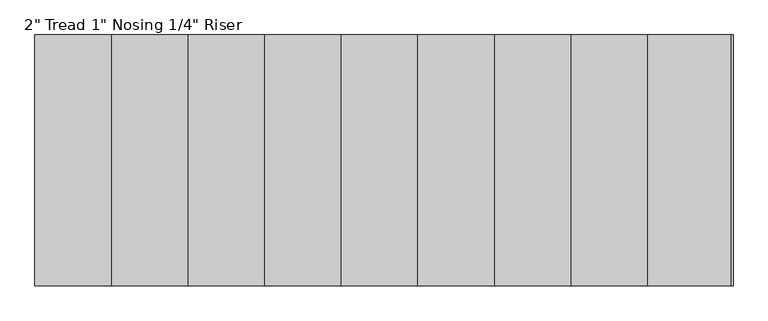
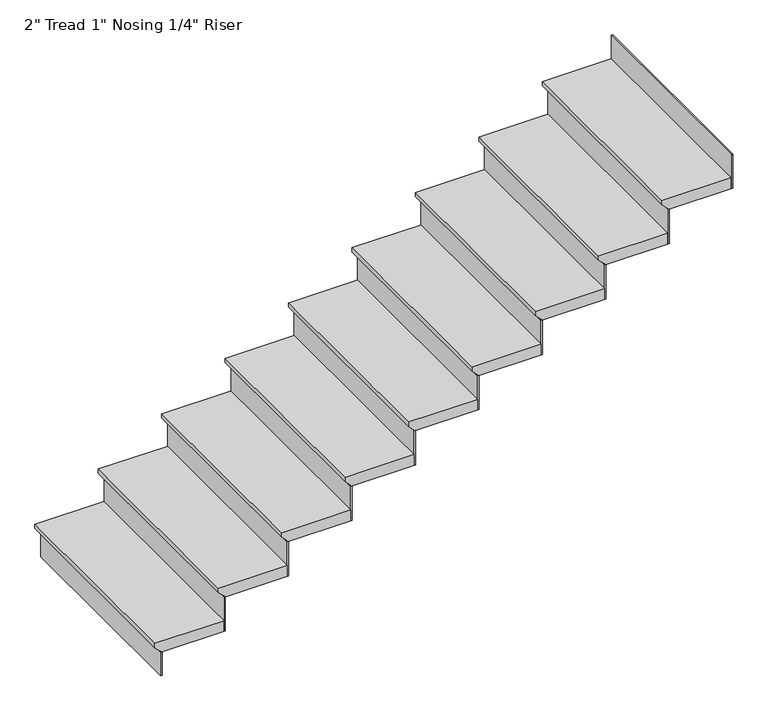
"""IFC4 building model written with IfcOpenShell, lengths in millimetres: stair flight geometry."""

from ifc_helpers import new_model, si_unit, origin, place, context, project, spatial, faceted_brep, source, transform, mapped, element, save


def stair_flight_922384ce(model_context):
    return source(origin(), model_context, "Body", "Brep", [
        faceted_brep([(-1591.1154463, -4737.3544725, 140.97), (-1591.1154463, -4737.3544725, 160.02), (-1591.1154463, -3822.9544725, 160.02), (-1591.1154463, -3822.9544725, 140.97), (-1565.7154463, -4737.3544725, 115.57), (-1565.7154463, -3822.9544725, 115.57), (-1286.3154463, -4737.3544725, 160.02), (-1286.3154463, -3822.9544725, 160.02), (-1565.7154463, -3822.9544725, 109.22), (-1286.3154463, -3822.9544725, 109.22), (-1286.3154463, -4737.3544725, 109.22), (-1565.7154463, -4737.3544725, 109.22)], [[[0, 1, 2, 3]], [[4, 0, 3, 5]], [[2, 1, 6, 7]], [[8, 9, 10, 11]], [[2, 7, 9, 8, 5, 3]], [[8, 11, 4, 5]], [[6, 1, 0, 4, 11, 10]], [[7, 6, 10, 9]]]),
        faceted_brep([(-1565.7154463, -4737.3544725, 109.22), (-1565.7154463, -4737.3544725, 0.0), (-1559.3654463, -4737.3544725, 0.0), (-1559.3654463, -4737.3544725, 109.22), (-1565.7154463, -3822.9544725, 109.22), (-1559.3654463, -3822.9544725, 109.22), (-1559.3654463, -3822.9544725, 0.0), (-1565.7154463, -3822.9544725, 0.0)], [[[0, 1, 2, 3]], [[4, 5, 6, 7]], [[1, 0, 4, 7]], [[2, 1, 7, 6]], [[3, 2, 6, 5]], [[0, 3, 5, 4]]]),
        faceted_brep([(-1286.3154463, -4737.3544725, 269.24), (-1286.3154463, -4737.3544725, 109.22), (-1279.9654463, -4737.3544725, 109.22), (-1279.9654463, -4737.3544725, 269.24), (-1286.3154463, -3822.9544725, 269.24), (-1279.9654463, -3822.9544725, 269.24), (-1279.9654463, -3822.9544725, 109.22), (-1286.3154463, -3822.9544725, 109.22)], [[[0, 1, 2, 3]], [[4, 5, 6, 7]], [[1, 0, 4, 7]], [[2, 1, 7, 6]], [[3, 2, 6, 5]], [[0, 3, 5, 4]]]),
        faceted_brep([(-1311.7154463, -3822.9544725, 320.04), (-1311.7154463, -4737.3544725, 320.04), (-1006.9154463, -4737.3544725, 320.04), (-1006.9154463, -3822.9544725, 320.04), (-1286.3154463, -3822.9544725, 269.24), (-1006.9154463, -3822.9544725, 269.24), (-1006.9154463, -4737.3544725, 269.24), (-1286.3154463, -4737.3544725, 269.24), (-1286.3154463, -3822.9544725, 275.59), (-1311.7154463, -3822.9544725, 300.99), (-1286.3154463, -4737.3544725, 275.59), (-1311.7154463, -4737.3544725, 300.99)], [[[0, 1, 2, 3]], [[4, 5, 6, 7]], [[0, 3, 5, 4, 8, 9]], [[4, 7, 10, 8]], [[2, 1, 11, 10, 7, 6]], [[3, 2, 6, 5]], [[11, 1, 0, 9]], [[10, 11, 9, 8]]]),
        faceted_brep([(-1006.9154463, -4737.3544725, 429.26), (-1006.9154463, -4737.3544725, 269.24), (-1000.5654463, -4737.3544725, 269.24), (-1000.5654463, -4737.3544725, 429.26), (-1006.9154463, -3822.9544725, 429.26), (-1000.5654463, -3822.9544725, 429.26), (-1000.5654463, -3822.9544725, 269.24), (-1006.9154463, -3822.9544725, 269.24)], [[[0, 1, 2, 3]], [[4, 5, 6, 7]], [[1, 0, 4, 7]], [[2, 1, 7, 6]], [[3, 2, 6, 5]], [[0, 3, 5, 4]]]),
        faceted_brep([(-1032.3154463, -3822.9544725, 480.06), (-1032.3154463, -4737.3544725, 480.06), (-727.5154463, -4737.3544725, 480.06), (-727.5154463, -3822.9544725, 480.06), (-1006.9154463, -3822.9544725, 429.26), (-727.5154463, -3822.9544725, 429.26), (-727.5154463, -4737.3544725, 429.26), (-1006.9154463, -4737.3544725, 429.26), (-1006.9154463, -3822.9544725, 435.61), (-1032.3154463, -3822.9544725, 461.01), (-1006.9154463, -4737.3544725, 435.61), (-1032.3154463, -4737.3544725, 461.01)], [[[0, 1, 2, 3]], [[4, 5, 6, 7]], [[0, 3, 5, 4, 8, 9]], [[4, 7, 10, 8]], [[2, 1, 11, 10, 7, 6]], [[3, 2, 6, 5]], [[11, 1, 0, 9]], [[10, 11, 9, 8]]]),
        faceted_brep([(-727.5154463, -4737.3544725, 589.28), (-727.5154463, -4737.3544725, 429.26), (-721.1654463, -4737.3544725, 429.26), (-721.1654463, -4737.3544725, 589.28), (-727.5154463, -3822.9544725, 589.28), (-721.1654463, -3822.9544725, 589.28), (-721.1654463, -3822.9544725, 429.26), (-727.5154463, -3822.9544725, 429.26)], [[[0, 1, 2, 3]], [[4, 5, 6, 7]], [[1, 0, 4, 7]], [[2, 1, 7, 6]], [[3, 2, 6, 5]], [[0, 3, 5, 4]]]),
        faceted_brep([(-752.9154463, -3822.9544725, 640.08), (-752.9154463, -4737.3544725, 640.08), (-448.1154463, -4737.3544725, 640.08), (-448.1154463, -3822.9544725, 640.08), (-727.5154463, -3822.9544725, 589.28), (-448.1154463, -3822.9544725, 589.28), (-448.1154463, -4737.3544725, 589.28), (-727.5154463, -4737.3544725, 589.28), (-727.5154463, -3822.9544725, 595.63), (-752.9154463, -3822.9544725, 621.03), (-727.5154463, -4737.3544725, 595.63), (-752.9154463, -4737.3544725, 621.03)], [[[0, 1, 2, 3]], [[4, 5, 6, 7]], [[0, 3, 5, 4, 8, 9]], [[4, 7, 10, 8]], [[2, 1, 11, 10, 7, 6]], [[3, 2, 6, 5]], [[11, 1, 0, 9]], [[10, 11, 9, 8]]]),
        faceted_brep([(-448.1154463, -4737.3544725, 749.3), (-448.1154463, -4737.3544725, 589.28), (-441.7654463, -4737.3544725, 589.28), (-441.7654463, -4737.3544725, 749.3), (-448.1154463, -3822.9544725, 749.3), (-441.7654463, -3822.9544725, 749.3), (-441.7654463, -3822.9544725, 589.28), (-448.1154463, -3822.9544725, 589.28)], [[[0, 1, 2, 3]], [[4, 5, 6, 7]], [[1, 0, 4, 7]], [[2, 1, 7, 6]], [[3, 2, 6, 5]], [[0, 3, 5, 4]]]),
        faceted_brep([(-473.5154463, -3822.9544725, 800.1), (-473.5154463, -4737.3544725, 800.1), (-168.7154463, -4737.3544725, 800.1), (-168.7154463, -3822.9544725, 800.1), (-448.1154463, -3822.9544725, 749.3), (-168.7154463, -3822.9544725, 749.3), (-168.7154463, -4737.3544725, 749.3), (-448.1154463, -4737.3544725, 749.3), (-448.1154463, -3822.9544725, 755.65), (-473.5154463, -3822.9544725, 781.05), (-448.1154463, -4737.3544725, 755.65), (-473.5154463, -4737.3544725, 781.05)], [[[0, 1, 2, 3]], [[4, 5, 6, 7]], [[0, 3, 5, 4, 8, 9]], [[4, 7, 10, 8]], [[2, 1, 11, 10, 7, 6]], [[3, 2, 6, 5]], [[11, 1, 0, 9]], [[10, 11, 9, 8]]]),
        faceted_brep([(-168.7154463, -4737.3544725, 909.32), (-168.7154463, -4737.3544725, 749.3), (-162.3654463, -4737.3544725, 749.3), (-162.3654463, -4737.3544725, 909.32), (-168.7154463, -3822.9544725, 909.32), (-162.3654463, -3822.9544725, 909.32), (-162.3654463, -3822.9544725, 749.3), (-168.7154463, -3822.9544725, 749.3)], [[[0, 1, 2, 3]], [[4, 5, 6, 7]], [[1, 0, 4, 7]], [[2, 1, 7, 6]], [[3, 2, 6, 5]], [[0, 3, 5, 4]]]),
        faceted_brep([(-194.1154463, -3822.9544725, 960.12), (-194.1154463, -4737.3544725, 960.12), (110.6845537, -4737.3544725, 960.12), (110.6845537, -3822.9544725, 960.12), (-168.7154463, -3822.9544725, 909.32), (110.6845537, -3822.9544725, 909.32), (110.6845537, -4737.3544725, 909.32), (-168.7154463, -4737.3544725, 909.32), (-168.7154463, -3822.9544725, 915.67), (-194.1154463, -3822.9544725, 941.07), (-168.7154463, -4737.3544725, 915.67), (-194.1154463, -4737.3544725, 941.07)], [[[0, 1, 2, 3]], [[4, 5, 6, 7]], [[0, 3, 5, 4, 8, 9]], [[4, 7, 10, 8]], [[2, 1, 11, 10, 7, 6]], [[3, 2, 6, 5]], [[11, 1, 0, 9]], [[10, 11, 9, 8]]]),
        faceted_brep([(110.6845537, -4737.3544725, 1069.34), (110.6845537, -4737.3544725, 909.32), (117.0345537, -4737.3544725, 909.32), (117.0345537, -4737.3544725, 1069.34), (110.6845537, -3822.9544725, 1069.34), (117.0345537, -3822.9544725, 1069.34), (117.0345537, -3822.9544725, 909.32), (110.6845537, -3822.9544725, 909.32)], [[[0, 1, 2, 3]], [[4, 5, 6, 7]], [[1, 0, 4, 7]], [[2, 1, 7, 6]], [[3, 2, 6, 5]], [[0, 3, 5, 4]]]),
        faceted_brep([(85.2845537, -3822.9544725, 1120.14), (85.2845537, -4737.3544725, 1120.14), (390.0845537, -4737.3544725, 1120.14), (390.0845537, -3822.9544725, 1120.14), (110.6845537, -3822.9544725, 1069.34), (390.0845537, -3822.9544725, 1069.34), (390.0845537, -4737.3544725, 1069.34), (110.6845537, -4737.3544725, 1069.34), (110.6845537, -3822.9544725, 1075.69), (85.2845537, -3822.9544725, 1101.09), (110.6845537, -4737.3544725, 1075.69), (85.2845537, -4737.3544725, 1101.09)], [[[0, 1, 2, 3]], [[4, 5, 6, 7]], [[0, 3, 5, 4, 8, 9]], [[4, 7, 10, 8]], [[2, 1, 11, 10, 7, 6]], [[3, 2, 6, 5]], [[11, 1, 0, 9]], [[10, 11, 9, 8]]]),
        faceted_brep([(390.0845537, -4737.3544725, 1229.36), (390.0845537, -4737.3544725, 1069.34), (396.4345537, -4737.3544725, 1069.34), (396.4345537, -4737.3544725, 1229.36), (390.0845537, -3822.9544725, 1229.36), (396.4345537, -3822.9544725, 1229.36), (396.4345537, -3822.9544725, 1069.34), (390.0845537, -3822.9544725, 1069.34)], [[[0, 1, 2, 3]], [[4, 5, 6, 7]], [[1, 0, 4, 7]], [[2, 1, 7, 6]], [[3, 2, 6, 5]], [[0, 3, 5, 4]]]),
        faceted_brep([(364.6845537, -3822.9544725, 1280.16), (364.6845537, -4737.3544725, 1280.16), (669.4845537, -4737.3544725, 1280.16), (669.4845537, -3822.9544725, 1280.16), (390.0845537, -3822.9544725, 1229.36), (669.4845537, -3822.9544725, 1229.36), (669.4845537, -4737.3544725, 1229.36), (390.0845537, -4737.3544725, 1229.36), (390.0845537, -3822.9544725, 1235.71), (364.6845537, -3822.9544725, 1261.11), (390.0845537, -4737.3544725, 1235.71), (364.6845537, -4737.3544725, 1261.11)], [[[0, 1, 2, 3]], [[4, 5, 6, 7]], [[0, 3, 5, 4, 8, 9]], [[4, 7, 10, 8]], [[2, 1, 11, 10, 7, 6]], [[3, 2, 6, 5]], [[11, 1, 0, 9]], [[10, 11, 9, 8]]]),
        faceted_brep([(948.8845537, -4737.3544725, 1549.4), (948.8845537, -4737.3544725, 1389.38), (955.2345537, -4737.3544725, 1389.38), (955.2345537, -4737.3544725, 1549.4), (948.8845537, -3822.9544725, 1549.4), (955.2345537, -3822.9544725, 1549.4), (955.2345537, -3822.9544725, 1389.38), (948.8845537, -3822.9544725, 1389.38)], [[[0, 1, 2, 3]], [[4, 5, 6, 7]], [[1, 0, 4, 7]], [[2, 1, 7, 6]], [[3, 2, 6, 5]], [[0, 3, 5, 4]]]),
        faceted_brep([(669.4845537, -4737.3544725, 1389.38), (669.4845537, -4737.3544725, 1229.36), (675.8345537, -4737.3544725, 1229.36), (675.8345537, -4737.3544725, 1389.38), (669.4845537, -3822.9544725, 1389.38), (675.8345537, -3822.9544725, 1389.38), (675.8345537, -3822.9544725, 1229.36), (669.4845537, -3822.9544725, 1229.36)], [[[0, 1, 2, 3]], [[4, 5, 6, 7]], [[1, 0, 4, 7]], [[2, 1, 7, 6]], [[3, 2, 6, 5]], [[0, 3, 5, 4]]]),
        faceted_brep([(948.8845537, -3822.9544725, 1440.18), (923.4845537, -3822.9544725, 1440.18), (644.0845537, -3822.9544725, 1440.18), (644.0845537, -4737.3544725, 1440.18), (948.8845537, -4737.3544725, 1440.18), (923.4845537, -3822.9544725, 1389.38), (948.8845537, -3822.9544725, 1389.38), (948.8845537, -4737.3544725, 1389.38), (669.4845537, -4737.3544725, 1389.38), (669.4845537, -3822.9544725, 1389.38), (669.4845537, -3822.9544725, 1395.73), (644.0845537, -3822.9544725, 1421.13), (669.4845537, -4737.3544725, 1395.73), (644.0845537, -4737.3544725, 1421.13)], [[[0, 1, 2, 3, 4]], [[5, 6, 7, 8, 9]], [[1, 0, 6, 5]], [[2, 1, 5, 9, 10, 11]], [[9, 8, 12, 10]], [[4, 3, 13, 12, 8, 7]], [[0, 4, 7, 6]], [[13, 3, 2, 11]], [[12, 13, 11, 10]]]),
    ])


if __name__ == "__main__":
    model = new_model("IFC4")
    model_context = context("Model", 3, world=origin())
    ifc_project = project(units=[si_unit("LENGTHUNIT", "METRE", prefix="MILLI")], contexts=[model_context])
    site = spatial("IfcSite", under=ifc_project)
    building = spatial("IfcBuilding", under=site)
    placement = place(None, origin())
    stair_flight_shape = stair_flight_922384ce(model_context)
    element("IfcStairFlight", 1, ObjectType="2\" Tread 1\" Nosing 1/4\" Riser", at=placement, inside=building, context=model_context, shape_type="MappedRepresentation", body=[
        mapped(stair_flight_shape, transform((0.0, 0.0, 0.0), x_axis=(1.0, 0.0, 0.0), y_axis=(0.0, 1.0, 0.0), z_axis=(0.0, 0.0, 1.0))),
    ])
    save(model, "model.ifc")
